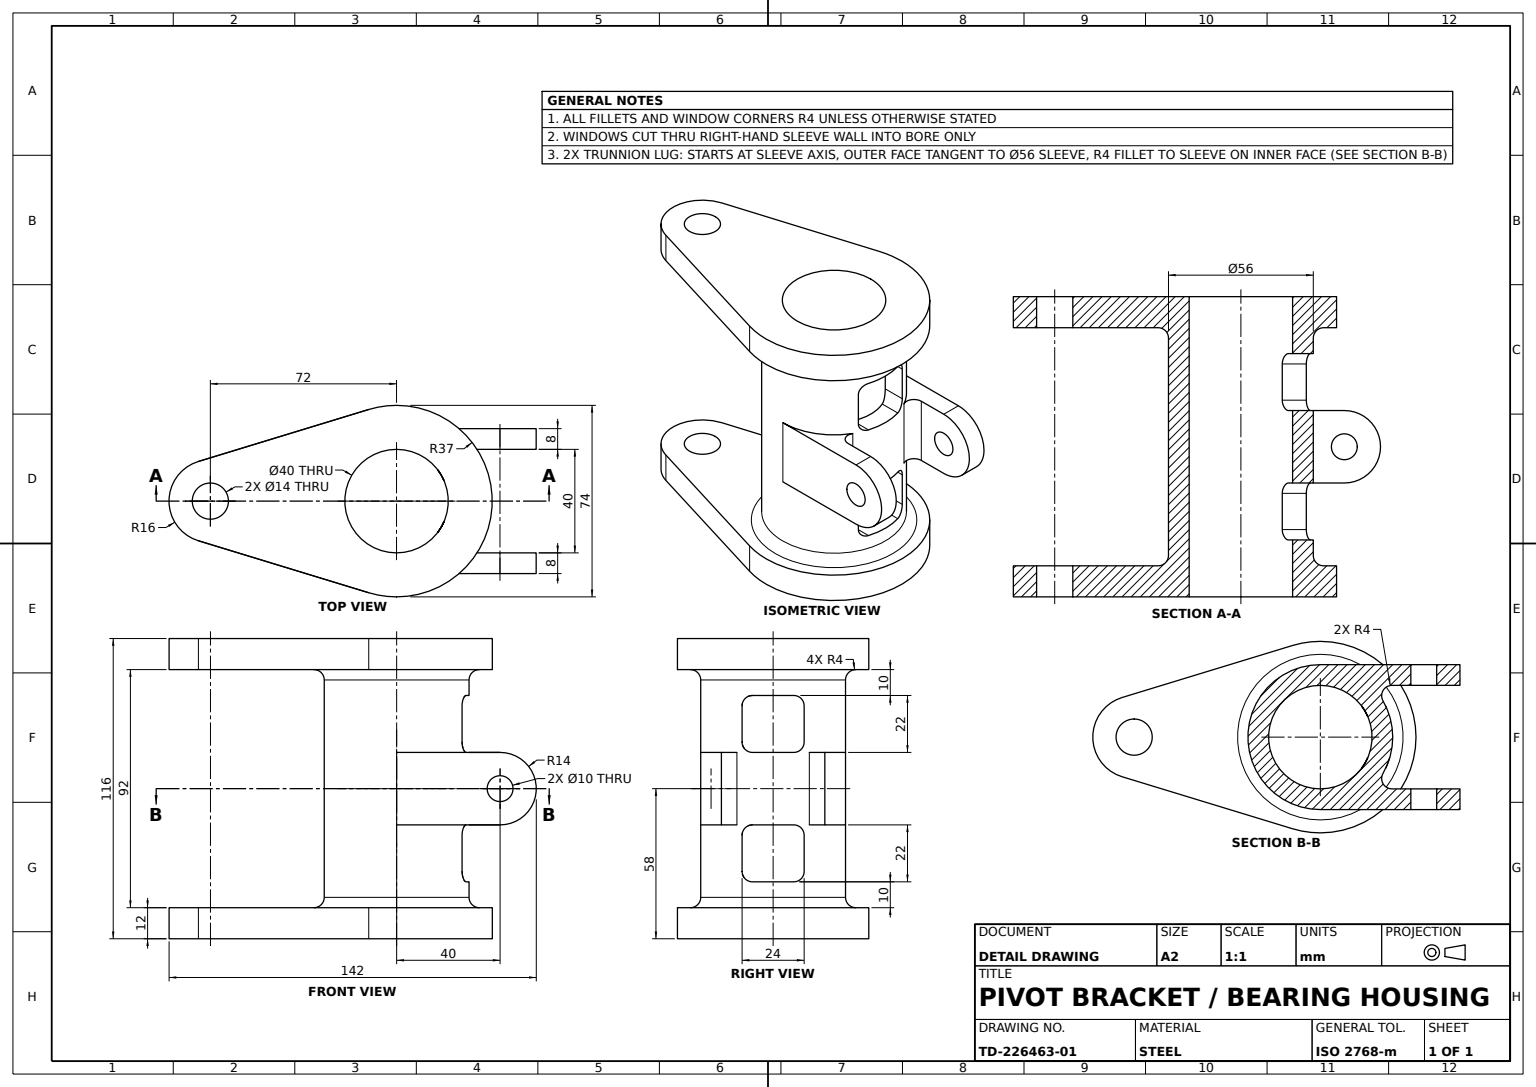
from build123d import *

# Parameters (mm, degrees)
LOWER_ARM_PROFILE_R    = 7
LOWER_ARM_PLATE_DEPTH  = 12
SLEEVE_PROFILE_56_R    = 28
SLEEVE_56_DEPTH        = 92
ARM_FILLETS_R4_R       = 4
TRUNNION_START         = 20
TRUNNION_LUG_PROFILE_R = 5
TRUNNION_LUG_DEPTH     = 8
LUG_FILLETS_R4_R       = 4
SLEEVE_WINDOWS_DEPTH   = 151.229823937
BORE_PROFILE_40_R      = 20
BORE_40_DEPTH          = 151.229823937


with BuildPart() as part:
    # Lower Arm Profile → Lower Arm Plate (new body)
    with BuildSketch(Plane(origin=(0, 0, 0), x_dir=(1, 0, 0), z_dir=(0, 1, 0))):
        with BuildLine():
            Line((-76.666666667, 15.304320378), (-10.791666667, 35.391240873))
            ThreePointArc((-10.791666667, 35.391240873), (37, 0), (-10.791666667, -35.391240873))
            Line((-10.791666667, -35.391240873), (-76.666666667, -15.304320378))
            ThreePointArc((-76.666666667, -15.304320378), (-88, 0), (-76.666666667, 15.304320378))
        make_face()
        with Locations(Location((-72, 0, 0), (0, 0, 270))):
            Circle(LOWER_ARM_PROFILE_R, mode=Mode.SUBTRACT)
    lower_arm_plate = extrude(amount=LOWER_ARM_PLATE_DEPTH)

    # Sleeve Profile Ø56 → Sleeve Ø56 (add)
    with BuildSketch(Plane(origin=(0, 12, 0), x_dir=(1, 0, 0), z_dir=(0, 1, 0))):
        with Locations(Location((0, 0, 0), (0, 0, 270))):
            Circle(SLEEVE_PROFILE_56_R)
    extrude(amount=SLEEVE_56_DEPTH)

    # Upper Arm Mirror: Lower Arm Plate across plane
    add(lower_arm_plate.mirror(Plane.ZX.offset(58)))

    # Arm Fillets R4
    arm_fillets_r4_edges = [part.edges().sort_by_distance(p)[0] for p in [
        (0, 12, -28),
        (0, 104, -28),
    ]]
    fillet(arm_fillets_r4_edges, radius=ARM_FILLETS_R4_R)

    # Trunnion Lug Profile → Trunnion Lug (add)
    with BuildSketch(Plane.XY.offset(TRUNNION_START)):
        with BuildLine():
            Line((0, 72), (40, 72))
            ThreePointArc((40, 72), (54, 58), (40, 44))
            Line((40, 44), (0, 44))
            Line((0, 44), (0, 72))
        make_face()
        with Locations((40, 58)):
            Circle(TRUNNION_LUG_PROFILE_R, mode=Mode.SUBTRACT)
    trunnion_lug = extrude(amount=TRUNNION_LUG_DEPTH)

    # Trunnion Lug Mirror: Trunnion Lug across plane
    add(trunnion_lug.mirror(Plane.XY))

    # Lug Fillets R4
    lug_fillets_r4_edges = [part.edges().sort_by_distance(p)[0] for p in [
        (19.595917942, 58, 20),
        (19.595917942, 58, -20),
    ]]
    fillet(lug_fillets_r4_edges, radius=LUG_FILLETS_R4_R)

    # Sleeve Window Profile → Sleeve Windows (cut, through all)
    with BuildSketch(Plane(origin=(0, 0, 0), x_dir=(0, 0, -1), z_dir=(1, 0, 0))):
        with BuildLine():
            Line((-8, 94), (8, 94))
            ThreePointArc((8, 94), (10.828427125, 92.828427125), (12, 90))
            Line((12, 90), (12, 76))
            ThreePointArc((12, 76), (10.828427125, 73.171572875), (8, 72))
            Line((8, 72), (-8, 72))
            ThreePointArc((-8, 72), (-10.828427125, 73.171572875), (-12, 76))
            Line((-12, 76), (-12, 90))
            ThreePointArc((-12, 90), (-10.828427125, 92.828427125), (-8, 94))
        make_face()
        with BuildLine():
            Line((-8, 22), (8, 22))
            ThreePointArc((8, 22), (10.828427125, 23.171572875), (12, 26))
            Line((12, 26), (12, 40))
            ThreePointArc((12, 40), (10.828427125, 42.828427125), (8, 44))
            Line((8, 44), (-8, 44))
            ThreePointArc((-8, 44), (-10.828427125, 42.828427125), (-12, 40))
            Line((-12, 40), (-12, 26))
            ThreePointArc((-12, 26), (-10.828427125, 23.171572875), (-8, 22))
        make_face()
    extrude(amount=SLEEVE_WINDOWS_DEPTH, mode=Mode.SUBTRACT)

    # Bore Profile Ø40 → Bore Ø40 (cut, through all)
    with BuildSketch(Plane(origin=(0, 116, 0), x_dir=(1, 0, 0), z_dir=(0, 1, 0))):
        with Locations(Location((0, 0, 0), (0, 0, 270))):
            Circle(BORE_PROFILE_40_R)
    extrude(amount=-BORE_40_DEPTH, mode=Mode.SUBTRACT)


solid = part.part
